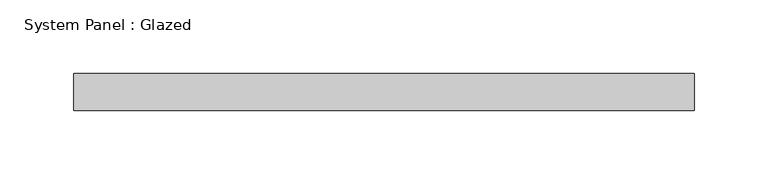
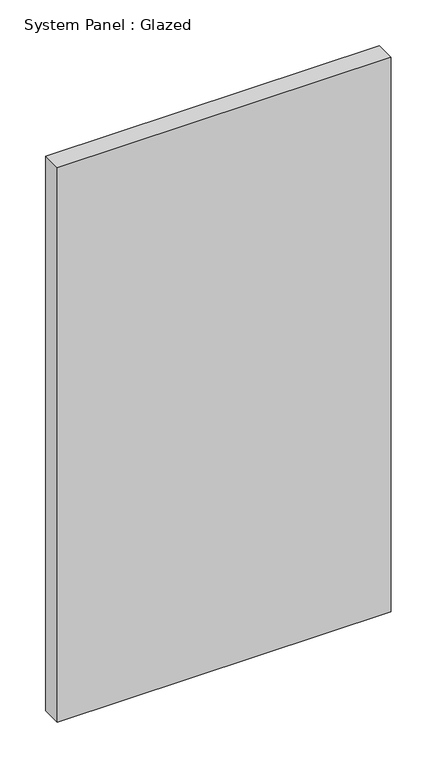
"""IFC4 building model written with IfcOpenShell, lengths in millimetres: plate geometry, System Panel : Glazed."""

from ifc_helpers import new_model, si_unit, origin, origin_with_axes, place, context, project, spatial, polyline, outline, extrude, source, transform, mapped, element, save


def system_panel_glazed_bba74dcb(model_context):
    return source(origin(), model_context, "Body", "SweptSolid", [
        extrude(outline(polyline([(209.7248465, 24.5), (-209.7248465, 24.5), (-209.7248465, 49.5), (209.7248465, 49.5), (209.7248465, 24.5)])), origin_with_axes(), (0.0, 0.0, 1.0), 736.6),
    ])


if __name__ == "__main__":
    model = new_model("IFC4")
    model_context = context("Model", 3, world=origin())
    ifc_project = project(units=[si_unit("LENGTHUNIT", "METRE", prefix="MILLI")], contexts=[model_context])
    site = spatial("IfcSite", under=ifc_project)
    building = spatial("IfcBuilding", under=site)
    placement = place(None, origin())
    system_panel_glazed_shape = system_panel_glazed_bba74dcb(model_context)
    element("IfcPlate", 1, ObjectType="System Panel : Glazed", at=placement, inside=building, context=model_context, shape_type="MappedRepresentation", body=[
        mapped(system_panel_glazed_shape, transform((0.0, 0.0, 0.0), x_axis=(1.0, 0.0, 0.0), y_axis=(0.0, 1.0, 0.0), z_axis=(0.0, 0.0, 1.0))),
    ])
    save(model, "model.ifc")

# Revit data of these elements
# Type "System Panel : Glazed"
#   Keynote = "H11"
#   Construction Type Id = "GSP4R"
#   Analytic Construction = "1/8 in Pilkington single glazing"
#   Visual Light Transmittance = 0.9
#   Solar Heat Gain Coefficient = 0.86
#   Heat Transfer Coefficient (U) = 6.7069 W/(m²·K)
#   Define Thermal Properties by = 1
# Element 1 (IfcPlate, "System Panel : Glazed")
#   Materials on its faces: "Glass"
# Materials
#   "Glass": class "Glass", colour RGB 0 128 192, transparency 0.9, Description = "Soda Lime Glass", Cost = 0
